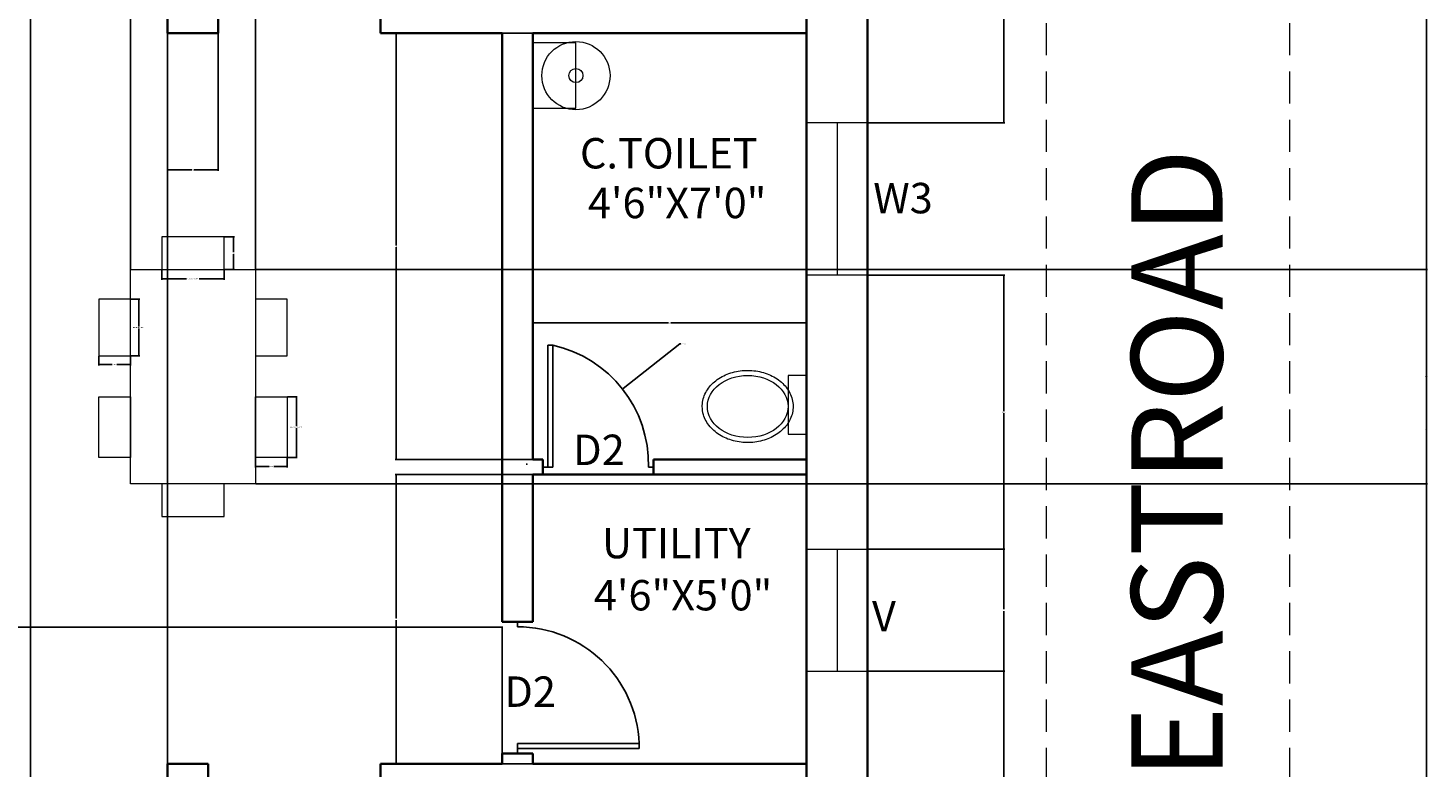
# Model space of a CAD drawing. Units: inches. Extents: x 2906 to 3403, y 1614 to 2150.
# Tile 3 of 4: x 3127 to 3403, y 1814 to 1960. Entities that reach past the tile are written whole.
import ezdxf

# ---------------------------------------------------------------- set-up
doc = ezdxf.new("R2010")
doc.units = ezdxf.units.IN
doc.linetypes.add('DASHED2', pattern=[9.525, 6.35, -3.175])
for name, color, linetype, lineweight in [('A-ANNO-DIMS', 2, 'Continuous', 18), ('A-ANNO-TEXT', 220, 'Continuous', 18), ('A-AREA-IDEN', 220, 'Continuous', 25), ('A-DOOR', 40, 'Continuous', 25), ('A-FLOR-FIXT', 121, 'Continuous', 18), ('A-FURN', 121, 'Continuous', 18), ('A-GLAZ', 2, 'Continuous', 18), ('A-WALL', 191, 'Continuous', 35), ('C-ROAD', 255, 'DASHED2', 18)]:
    doc.layers.add(name, color=color, linetype=linetype, lineweight=lineweight)
doc.styles.get("Standard").update_dxf_attribs({"font": 'arial.ttf'})
doc.dimstyles.get("Standard").update_dxf_attribs({"dimtxt": 0.18, "dimasz": 0.18, "dimexe": 0.18, "dimexo": 0.0625, "dimgap": 0.09, "dimtad": 0, "dimtih": 1, "dimtoh": 1, "dimdec": 4, "dimzin": 0, "dimdsep": 46, "dimtxsty": 'Standard', "dimcen": 0.09, "dimadec": 0, "dimazin": 0, "dimtfac": 1, "dimtdec": 4, "dimtofl": 0, "dimtmove": 0, "dimatfit": 3, "dimfxl": 1, "dimtolj": 1, "dimtzin": 0, "dimarcsym": 0})

# ---------------------------------------------------------------- blocks, each defined once
blk = doc.blocks.new('WINDOW-30')
for p, q in [((0, 12), (0, 0)), ((30, 12), (30, 0)), ((0, 6), (30, 6))]:
    blk.add_line(p, q)
blk = doc.blocks.new('WC-FLOOR')
blk.add_lwpolyline([(20.57, 13.25), (16.9, 13.25), (16.9, 1.66), (20.57, 1.66)], close=True)
blk.add_ellipse((8.95, 7.12), major_axis=(-7.95, 0), ratio=0.769471)
blk.add_open_spline([(0, 7.12), (0, 6.57), (0.08, 6.02), (0.48, 4.65), (0.93, 3.84), (2.12, 2.43), (2.86, 1.82), (4.56, 0.85), (5.51, 0.49), (7.5, 0.04), (8.54, -0.04), (10.6, 0.07), (11.62, 0.27), (13.52, 0.93), (14.4, 1.4), (15.92, 2.56), (16.56, 3.25), (17.49, 4.8), (17.78, 5.66), (17.96, 7.41), (17.85, 8.3), (17.23, 9.97), (16.74, 10.74), (15.46, 12.09), (14.67, 12.67), (12.92, 13.56), (11.94, 13.88), (9.93, 14.24), (8.88, 14.28), (6.83, 14.08), (5.83, 13.84), (3.97, 13.1), (3.12, 12.59), (1.68, 11.37), (1.09, 10.64), (0.26, 9.05), (0.03, 8.17), (0, 7.24), (0, 7.18), (0, 7.12)], degree=3, knots=[0, 0, 0, 0, 0.221105, 0.221105, 0.576279, 0.576279, 0.931454, 0.931454, 1.286628, 1.286628, 1.641803, 1.641803, 1.996977, 1.996977, 2.352152, 2.352152, 2.707326, 2.707326, 3.062501, 3.062501, 3.417675, 3.417675, 3.77285, 3.77285, 4.128024, 4.128024, 4.483198, 4.483198, 4.838373, 4.838373, 5.193547, 5.193547, 5.548722, 5.548722, 5.903896, 5.903896, 6.259071, 6.259071, 6.283185, 6.283185, 6.283185, 6.283185])
blk = doc.blocks.new('LAVATORY-WALL')
blk.add_lwpolyline([(15.24, 13.17), (6.72, 13.17), (6.72, 0.27), (15.24, 0.27)], close=True)
for radius in [6.72, 1.39]:
    blk.add_circle((6.72, 6.72), radius)
blk = doc.blocks.new('DINING-CHAIR-END')
blk.add_lwpolyline([(0, 0), (12.31, 0), (12.31, 6.47), (0, 6.47)], close=True)
blk = doc.blocks.new('DINING-CHAIR-SIDE-A')
blk.add_lwpolyline([(6.24, 11.19), (0, 11.19), (0, 0), (6.24, 0)], close=True)
blk = doc.blocks.new('DINING-CHAIR-SIDE-B')
blk.add_lwpolyline([(6.24, 0), (0, 0), (0, 11.97), (6.24, 11.97)], close=True)
blk = doc.blocks.new('*D34')
at = {"layer": 'A-ANNO-DIMS', "color": 0, "lineweight": -2, "transparency": 16777216}
for p, q in [((3153.49, 1912.61), (3153.49, 1910.65)), ((3153.67, 1910.83), (3158.4, 1910.83)), ((3165.63, 1910.83), (3160.9, 1910.83)), ((3165.81, 1912.61), (3165.81, 1910.65))]:
    blk.add_line(p, q, dxfattribs=at)
at = {"layer": 'A-ANNO-DIMS', "color": 0, "transparency": 16777216}
for points in [[(3153.67, 1910.86), (3153.67, 1910.8), (3153.49, 1910.83)], [(3165.63, 1910.86), (3165.63, 1910.8), (3165.81, 1910.83)]]:
    blk.add_solid(points, dxfattribs=at)
at = {"layer": 'Defpoints', "color": 0, "transparency": 16777216}
for p in [(3153.49, 1912.68), (3165.81, 1912.68), (3165.81, 1910.83)]:
    blk.add_point(p, dxfattribs=at)
at = {"layer": 'A-ANNO-DIMS', "color": 0, "transparency": 16777216, "insert": (3159.65, 1910.83), "char_height": 0.18, "attachment_point": 5}
blk.add_mtext('\\A1;END CHAIR 12 TYP.', dxfattribs=at)
blk = doc.blocks.new('*D35')
at = {"layer": 'A-ANNO-DIMS', "color": 0, "lineweight": -2, "transparency": 16777216}
for p, q in [((3165.87, 1919.15), (3167.83, 1919.15)), ((3167.65, 1918.97), (3167.65, 1916.1)), ((3167.65, 1912.86), (3167.65, 1915.73)), ((3165.87, 1912.68), (3167.83, 1912.68))]:
    blk.add_line(p, q, dxfattribs=at)
at = {"layer": 'A-ANNO-DIMS', "color": 0, "transparency": 16777216}
for points in [[(3167.62, 1918.97), (3167.68, 1918.97), (3167.65, 1919.15)], [(3167.62, 1912.86), (3167.68, 1912.86), (3167.65, 1912.68)]]:
    blk.add_solid(points, dxfattribs=at)
at = {"layer": 'Defpoints', "color": 0, "transparency": 16777216}
for p in [(3165.81, 1919.15), (3167.65, 1919.15), (3165.81, 1912.68)]:
    blk.add_point(p, dxfattribs=at)
at = {"layer": 'A-ANNO-DIMS', "color": 0, "transparency": 16777216, "insert": (3167.65, 1915.91), "char_height": 0.18, "attachment_point": 5}
blk.add_mtext('\\A1;6 TYP.', dxfattribs=at)
blk = doc.blocks.new('*D36')
at = {"layer": 'A-ANNO-DIMS', "color": 0, "lineweight": -2, "transparency": 16777216}
for p, q in [((3147.39, 1906.84), (3149.18, 1906.84)), ((3149, 1906.66), (3149, 1901.43)), ((3149, 1895.83), (3149, 1901.06)), ((3147.39, 1895.65), (3149.18, 1895.65))]:
    blk.add_line(p, q, dxfattribs=at)
at = {"layer": 'A-ANNO-DIMS', "color": 0, "transparency": 16777216}
for points in [[(3148.97, 1906.66), (3149.03, 1906.66), (3149, 1906.84)], [(3148.97, 1895.83), (3149.03, 1895.83), (3149, 1895.65)]]:
    blk.add_solid(points, dxfattribs=at)
at = {"layer": 'Defpoints', "color": 0, "transparency": 16777216}
for p in [(3147.32, 1906.84), (3149, 1906.84), (3147.32, 1895.65)]:
    blk.add_point(p, dxfattribs=at)
at = {"layer": 'A-ANNO-DIMS', "color": 0, "transparency": 16777216, "insert": (3149, 1901.25), "char_height": 0.18, "attachment_point": 5}
blk.add_mtext('\\A1;SIDE CHAIR A 11 TYP.', dxfattribs=at)
blk = doc.blocks.new('*D37')
at = {"layer": 'A-ANNO-DIMS', "color": 0, "lineweight": -2, "transparency": 16777216}
for p, q in [((3141.08, 1895.59), (3141.08, 1893.79)), ((3141.26, 1893.97), (3143.75, 1893.97)), ((3147.14, 1893.97), (3144.66, 1893.97)), ((3147.32, 1895.59), (3147.32, 1893.79))]:
    blk.add_line(p, q, dxfattribs=at)
at = {"layer": 'A-ANNO-DIMS', "color": 0, "transparency": 16777216}
for points in [[(3141.26, 1894), (3141.26, 1893.94), (3141.08, 1893.97)], [(3147.14, 1894), (3147.14, 1893.94), (3147.32, 1893.97)]]:
    blk.add_solid(points, dxfattribs=at)
at = {"layer": 'Defpoints', "color": 0, "transparency": 16777216}
for p in [(3141.08, 1895.65), (3147.32, 1895.65), (3147.32, 1893.97)]:
    blk.add_point(p, dxfattribs=at)
at = {"layer": 'A-ANNO-DIMS', "color": 0, "transparency": 16777216, "insert": (3144.2, 1893.97), "char_height": 0.18, "attachment_point": 5}
blk.add_mtext('\\A1;6 TYP.', dxfattribs=at)
blk = doc.blocks.new('*D38')
at = {"layer": 'A-ANNO-DIMS', "color": 0, "lineweight": -2, "transparency": 16777216}
for p, q in [((3178.3, 1887.61), (3180.22, 1887.61)), ((3180.04, 1887.43), (3180.04, 1881.8)), ((3180.04, 1875.81), (3180.04, 1881.44)), ((3178.3, 1875.63), (3180.22, 1875.63))]:
    blk.add_line(p, q, dxfattribs=at)
at = {"layer": 'A-ANNO-DIMS', "color": 0, "transparency": 16777216}
for points in [[(3180.01, 1887.43), (3180.07, 1887.43), (3180.04, 1887.61)], [(3180.01, 1875.81), (3180.07, 1875.81), (3180.04, 1875.63)]]:
    blk.add_solid(points, dxfattribs=at)
at = {"layer": 'Defpoints', "color": 0, "transparency": 16777216}
for p in [(3178.24, 1887.61), (3180.04, 1887.61), (3178.24, 1875.63)]:
    blk.add_point(p, dxfattribs=at)
at = {"layer": 'A-ANNO-DIMS', "color": 0, "transparency": 16777216, "insert": (3180.04, 1881.62), "char_height": 0.18, "attachment_point": 5}
blk.add_mtext('\\A1;SIDE CHAIR B 12 TYP.', dxfattribs=at)
blk = doc.blocks.new('*D39')
at = {"layer": 'A-ANNO-DIMS', "color": 0, "lineweight": -2, "transparency": 16777216}
for p, q in [((3172, 1875.57), (3172, 1873.66)), ((3178.24, 1875.57), (3178.24, 1873.66)), ((3172.18, 1873.84), (3174.66, 1873.84)), ((3178.06, 1873.84), (3175.58, 1873.84))]:
    blk.add_line(p, q, dxfattribs=at)
at = {"layer": 'A-ANNO-DIMS', "color": 0, "transparency": 16777216}
for points in [[(3172.18, 1873.87), (3172.18, 1873.81), (3172, 1873.84)], [(3178.06, 1873.87), (3178.06, 1873.81), (3178.24, 1873.84)]]:
    blk.add_solid(points, dxfattribs=at)
at = {"layer": 'Defpoints', "color": 0, "transparency": 16777216}
for p in [(3172, 1875.63), (3178.24, 1875.63), (3178.24, 1873.84)]:
    blk.add_point(p, dxfattribs=at)
at = {"layer": 'A-ANNO-DIMS', "color": 0, "transparency": 16777216, "insert": (3175.12, 1873.84), "char_height": 0.18, "attachment_point": 5}
blk.add_mtext('\\A1;6 TYP.', dxfattribs=at)
blk = doc.blocks.new('*D41')
at = {"layer": 'A-ANNO-DIMS', "color": 0, "lineweight": -2, "transparency": 16777216}
for p, q in [((3292.7, 2121.25), (3403.01, 2121.25)), ((3402.83, 2121.07), (3402.83, 1881.44)), ((3402.83, 1641.43), (3402.83, 1881.07)), ((3292.7, 1641.25), (3403.01, 1641.25))]:
    blk.add_line(p, q, dxfattribs=at)
at = {"layer": 'A-ANNO-DIMS', "color": 0, "transparency": 16777216}
for points in [[(3402.8, 2121.07), (3402.86, 2121.07), (3402.83, 2121.25)], [(3402.8, 1641.43), (3402.86, 1641.43), (3402.83, 1641.25)]]:
    blk.add_solid(points, dxfattribs=at)
at = {"layer": 'Defpoints', "color": 0, "transparency": 16777216}
for p in [(3292.63, 2121.25), (3402.83, 2121.25), (3292.63, 1641.25)]:
    blk.add_point(p, dxfattribs=at)
at = {"layer": 'A-ANNO-DIMS', "color": 0, "transparency": 16777216, "insert": (3402.83, 1881.25), "char_height": 0.18, "attachment_point": 5}
blk.add_mtext('\\A1;480', dxfattribs=at)
blk = doc.blocks.new('*D59')
at = {"layer": 'A-ANNO-DIMS', "color": 0, "lineweight": -2, "transparency": 16777216}
for p, q in [((3226.63, 1875.32), (3226.63, 1902.33)), ((3226.81, 1902.15), (3253.41, 1902.15)), ((3280.45, 1902.15), (3253.85, 1902.15)), ((3280.63, 1875.32), (3280.63, 1902.33))]:
    blk.add_line(p, q, dxfattribs=at)
at = {"layer": 'A-ANNO-DIMS', "color": 0, "transparency": 16777216}
for points in [[(3226.81, 1902.18), (3226.81, 1902.12), (3226.63, 1902.15)], [(3280.45, 1902.18), (3280.45, 1902.12), (3280.63, 1902.15)]]:
    blk.add_solid(points, dxfattribs=at)
at = {"layer": 'Defpoints', "color": 0, "transparency": 16777216}
for p in [(3280.63, 1902.15), (3226.63, 1875.25), (3280.63, 1875.25)]:
    blk.add_point(p, dxfattribs=at)
at = {"layer": 'A-ANNO-DIMS', "color": 0, "transparency": 16777216, "insert": (3253.63, 1902.15), "char_height": 0.18, "attachment_point": 5}
blk.add_mtext('\\A1;54', dxfattribs=at)
blk = doc.blocks.new('*D62')
at = {"layer": 'A-ANNO-DIMS', "color": 0, "lineweight": -2, "transparency": 16777216}
for p, q in [((3226.57, 1872.25), (3199.55, 1872.25)), ((3199.73, 1872.07), (3199.73, 1843.94)), ((3199.73, 1815.43), (3199.73, 1843.57)), ((3226.57, 1815.25), (3199.55, 1815.25))]:
    blk.add_line(p, q, dxfattribs=at)
at = {"layer": 'A-ANNO-DIMS', "color": 0, "transparency": 16777216}
for points in [[(3199.7, 1872.07), (3199.76, 1872.07), (3199.73, 1872.25)], [(3199.7, 1815.43), (3199.76, 1815.43), (3199.73, 1815.25)]]:
    blk.add_solid(points, dxfattribs=at)
at = {"layer": 'Defpoints', "color": 0, "transparency": 16777216}
for p in [(3199.73, 1872.25), (3226.63, 1872.25), (3226.63, 1815.25)]:
    blk.add_point(p, dxfattribs=at)
at = {"layer": 'A-ANNO-DIMS', "color": 0, "transparency": 16777216, "insert": (3199.73, 1843.75), "char_height": 0.18, "attachment_point": 5}
blk.add_mtext('\\A1;57', dxfattribs=at)
blk = doc.blocks.new('*D63')
at = {"layer": 'A-ANNO-DIMS', "color": 0, "lineweight": -2, "transparency": 16777216}
for p, q in [((3226.57, 1959.25), (3199.55, 1959.25)), ((3199.73, 1959.07), (3199.73, 1917.44)), ((3199.73, 1875.43), (3199.73, 1917.07)), ((3226.57, 1875.25), (3199.55, 1875.25))]:
    blk.add_line(p, q, dxfattribs=at)
at = {"layer": 'A-ANNO-DIMS', "color": 0, "transparency": 16777216}
for points in [[(3199.7, 1959.07), (3199.76, 1959.07), (3199.73, 1959.25)], [(3199.7, 1875.43), (3199.76, 1875.43), (3199.73, 1875.25)]]:
    blk.add_solid(points, dxfattribs=at)
at = {"layer": 'Defpoints', "color": 0, "transparency": 16777216}
for p in [(3199.73, 1959.25), (3226.63, 1959.25), (3226.63, 1875.25)]:
    blk.add_point(p, dxfattribs=at)
at = {"layer": 'A-ANNO-DIMS', "color": 0, "transparency": 16777216, "insert": (3199.73, 1917.25), "char_height": 0.18, "attachment_point": 5}
blk.add_mtext('\\A1;84', dxfattribs=at)
blk = doc.blocks.new('*D65')
at = {"layer": 'A-ANNO-DIMS', "color": 0, "lineweight": -2, "transparency": 16777216}
for p, q in [((2944.63, 1815.32), (2944.63, 1842.33)), ((2944.81, 1842.15), (3082.34, 1842.15)), ((3220.45, 1842.15), (3082.92, 1842.15)), ((3220.63, 1815.32), (3220.63, 1842.33))]:
    blk.add_line(p, q, dxfattribs=at)
at = {"layer": 'A-ANNO-DIMS', "color": 0, "transparency": 16777216}
for points in [[(2944.81, 1842.18), (2944.81, 1842.12), (2944.63, 1842.15)], [(3220.45, 1842.18), (3220.45, 1842.12), (3220.63, 1842.15)]]:
    blk.add_solid(points, dxfattribs=at)
at = {"layer": 'Defpoints', "color": 0, "transparency": 16777216}
for p in [(3220.63, 1842.15), (2944.63, 1815.25), (3220.63, 1815.25)]:
    blk.add_point(p, dxfattribs=at)
at = {"layer": 'A-ANNO-DIMS', "color": 0, "transparency": 16777216, "insert": (3082.63, 1842.15), "char_height": 0.18, "attachment_point": 5}
blk.add_mtext('\\A1;276', dxfattribs=at)
blk = doc.blocks.new('*D66')
at = {"layer": 'A-ANNO-DIMS', "color": 0, "lineweight": -2, "transparency": 16777216}
for p, q in [((3292.7, 2121.25), (3319.71, 2121.25)), ((3319.53, 2121.07), (3319.53, 2031.6)), ((3319.53, 1941.76), (3319.53, 2031.24)), ((3292.7, 1941.58), (3319.71, 1941.58))]:
    blk.add_line(p, q, dxfattribs=at)
at = {"layer": 'A-ANNO-DIMS', "color": 0, "transparency": 16777216}
for points in [[(3319.5, 2121.07), (3319.56, 2121.07), (3319.53, 2121.25)], [(3319.5, 1941.76), (3319.56, 1941.76), (3319.53, 1941.58)]]:
    blk.add_solid(points, dxfattribs=at)
at = {"layer": 'Defpoints', "color": 0, "transparency": 16777216}
for p in [(3292.63, 2121.25), (3292.63, 1941.58), (3319.53, 1941.58)]:
    blk.add_point(p, dxfattribs=at)
at = {"layer": 'A-ANNO-DIMS', "color": 0, "transparency": 16777216, "insert": (3319.53, 2031.42), "char_height": 0.18, "attachment_point": 5}
blk.add_mtext('\\A1;179.67', dxfattribs=at)
blk = doc.blocks.new('*D67')
at = {"layer": 'A-ANNO-DIMS', "color": 0, "lineweight": -2, "transparency": 16777216}
for p, q in [((3292.7, 1911.58), (3319.71, 1911.58)), ((3319.53, 1911.4), (3319.53, 1884.74)), ((3319.53, 1857.71), (3319.53, 1884.37)), ((3292.7, 1857.53), (3319.71, 1857.53))]:
    blk.add_line(p, q, dxfattribs=at)
at = {"layer": 'A-ANNO-DIMS', "color": 0, "transparency": 16777216}
for points in [[(3319.5, 1911.4), (3319.56, 1911.4), (3319.53, 1911.58)], [(3319.5, 1857.71), (3319.56, 1857.71), (3319.53, 1857.53)]]:
    blk.add_solid(points, dxfattribs=at)
at = {"layer": 'Defpoints', "color": 0, "transparency": 16777216}
for p in [(3292.63, 1911.58), (3292.63, 1857.53), (3319.53, 1857.53)]:
    blk.add_point(p, dxfattribs=at)
at = {"layer": 'A-ANNO-DIMS', "color": 0, "transparency": 16777216, "insert": (3319.53, 1884.56), "char_height": 0.18, "attachment_point": 5}
blk.add_mtext('\\A1;54.05', dxfattribs=at)
blk = doc.blocks.new('*D68')
at = {"layer": 'A-ANNO-DIMS', "color": 0, "lineweight": -2, "transparency": 16777216}
for p, q in [((3292.7, 1857.53), (3319.71, 1857.53)), ((3319.53, 1857.35), (3319.53, 1845.71)), ((3319.53, 1833.71), (3319.53, 1845.35)), ((3292.7, 1833.53), (3319.71, 1833.53))]:
    blk.add_line(p, q, dxfattribs=at)
at = {"layer": 'A-ANNO-DIMS', "color": 0, "transparency": 16777216}
for points in [[(3319.5, 1857.35), (3319.56, 1857.35), (3319.53, 1857.53)], [(3319.5, 1833.71), (3319.56, 1833.71), (3319.53, 1833.53)]]:
    blk.add_solid(points, dxfattribs=at)
at = {"layer": 'Defpoints', "color": 0, "transparency": 16777216}
for p in [(3292.63, 1857.53), (3292.63, 1833.53), (3319.53, 1833.53)]:
    blk.add_point(p, dxfattribs=at)
at = {"layer": 'A-ANNO-DIMS', "color": 0, "transparency": 16777216, "insert": (3319.53, 1845.53), "char_height": 0.18, "attachment_point": 5}
blk.add_mtext('\\A1;24', dxfattribs=at)
blk = doc.blocks.new('*D69')
at = {"layer": 'A-ANNO-DIMS', "color": 0, "lineweight": -2, "transparency": 16777216}
for p, q in [((3292.7, 1833.53), (3319.71, 1833.53)), ((3319.53, 1833.35), (3319.53, 1804.89)), ((3319.53, 1776.07), (3319.53, 1804.53)), ((3292.7, 1775.89), (3319.71, 1775.89))]:
    blk.add_line(p, q, dxfattribs=at)
at = {"layer": 'A-ANNO-DIMS', "color": 0, "transparency": 16777216}
for points in [[(3319.5, 1833.35), (3319.56, 1833.35), (3319.53, 1833.53)], [(3319.5, 1776.07), (3319.56, 1776.07), (3319.53, 1775.89)]]:
    blk.add_solid(points, dxfattribs=at)
at = {"layer": 'Defpoints', "color": 0, "transparency": 16777216}
for p in [(3292.63, 1833.53), (3292.63, 1775.89), (3319.53, 1775.89)]:
    blk.add_point(p, dxfattribs=at)
at = {"layer": 'A-ANNO-DIMS', "color": 0, "transparency": 16777216, "insert": (3319.53, 1804.71), "char_height": 0.18, "attachment_point": 5}
blk.add_mtext('\\A1;57.63', dxfattribs=at)
blk = doc.blocks.new('*D72')
at = {"layer": 'A-ANNO-DIMS', "color": 0, "lineweight": -2, "transparency": 16777216}
for p, q in [((3154.63, 1959.19), (3154.63, 1932.17)), ((3164.63, 1959.19), (3164.63, 1932.17)), ((3154.81, 1932.35), (3159.42, 1932.35)), ((3164.45, 1932.35), (3159.84, 1932.35))]:
    blk.add_line(p, q, dxfattribs=at)
at = {"layer": 'A-ANNO-DIMS', "color": 0, "transparency": 16777216}
for points in [[(3154.81, 1932.38), (3154.81, 1932.32), (3154.63, 1932.35)], [(3164.45, 1932.38), (3164.45, 1932.32), (3164.63, 1932.35)]]:
    blk.add_solid(points, dxfattribs=at)
at = {"layer": 'Defpoints', "color": 0, "transparency": 16777216}
for p in [(3154.63, 1959.25), (3164.63, 1959.25), (3154.63, 1932.35)]:
    blk.add_point(p, dxfattribs=at)
at = {"layer": 'A-ANNO-DIMS', "color": 0, "transparency": 16777216, "insert": (3159.63, 1932.35), "char_height": 0.18, "attachment_point": 5}
blk.add_mtext('\\A1;10', dxfattribs=at)
blk = doc.blocks.new('*D75')
at = {"layer": 'A-ANNO-DIMS', "color": 0, "lineweight": -2, "transparency": 16777216}
for p, q in [((3127.63, 2013.19), (3127.63, 1613.51)), ((3154.63, 2013.19), (3154.63, 1613.51)), ((3127.81, 1613.69), (3140.91, 1613.69)), ((3154.45, 1613.69), (3141.35, 1613.69))]:
    blk.add_line(p, q, dxfattribs=at)
at = {"layer": 'A-ANNO-DIMS', "color": 0, "transparency": 16777216}
for points in [[(3127.81, 1613.72), (3127.81, 1613.66), (3127.63, 1613.69)], [(3154.45, 1613.72), (3154.45, 1613.66), (3154.63, 1613.69)]]:
    blk.add_solid(points, dxfattribs=at)
at = {"layer": 'Defpoints', "color": 0, "transparency": 16777216}
for p in [(3127.63, 2013.25), (3154.63, 2013.25), (3154.63, 1613.69)]:
    blk.add_point(p, dxfattribs=at)
at = {"layer": 'A-ANNO-DIMS', "color": 0, "transparency": 16777216, "insert": (3141.13, 1613.69), "char_height": 0.18, "attachment_point": 5}
blk.add_mtext('\\A1;27', dxfattribs=at)
blk = doc.blocks.new('*D78')
at = {"layer": 'A-ANNO-DIMS', "color": 0, "lineweight": -2, "transparency": 16777216}
for p, q in [((3147.32, 1912.74), (3147.32, 2149.96)), ((3147.5, 2149.78), (3159.2, 2149.78)), ((3171.82, 2149.78), (3160.13, 2149.78)), ((3172, 1912.74), (3172, 2149.96))]:
    blk.add_line(p, q, dxfattribs=at)
at = {"layer": 'A-ANNO-DIMS', "color": 0, "transparency": 16777216}
for points in [[(3147.5, 2149.81), (3147.5, 2149.75), (3147.32, 2149.78)], [(3171.82, 2149.81), (3171.82, 2149.75), (3172, 2149.78)]]:
    blk.add_solid(points, dxfattribs=at)
at = {"layer": 'Defpoints', "color": 0, "transparency": 16777216}
for p in [(3172, 2149.78), (3147.32, 1912.68), (3172, 1912.68)]:
    blk.add_point(p, dxfattribs=at)
at = {"layer": 'A-ANNO-DIMS', "color": 0, "transparency": 16777216, "insert": (3159.66, 2149.78), "char_height": 0.18, "attachment_point": 5}
blk.add_mtext('\\A1;24.675', dxfattribs=at)
blk = doc.blocks.new('*D79')
at = {"layer": 'A-ANNO-DIMS', "color": 0, "lineweight": -2, "transparency": 16777216}
for p, q in [((3172.06, 1912.68), (3403.01, 1912.68)), ((3402.83, 1912.5), (3402.83, 1891.75)), ((3402.83, 1870.64), (3402.83, 1891.39)), ((3172.06, 1870.46), (3403.01, 1870.46))]:
    blk.add_line(p, q, dxfattribs=at)
at = {"layer": 'A-ANNO-DIMS', "color": 0, "transparency": 16777216}
for points in [[(3402.8, 1912.5), (3402.86, 1912.5), (3402.83, 1912.68)], [(3402.8, 1870.64), (3402.86, 1870.64), (3402.83, 1870.46)]]:
    blk.add_solid(points, dxfattribs=at)
at = {"layer": 'Defpoints', "color": 0, "transparency": 16777216}
for p in [(3172, 1912.68), (3402.83, 1912.68), (3172, 1870.46)]:
    blk.add_point(p, dxfattribs=at)
at = {"layer": 'A-ANNO-DIMS', "color": 0, "transparency": 16777216, "insert": (3402.83, 1891.57), "char_height": 0.18, "attachment_point": 5}
blk.add_mtext('\\A1;42.22', dxfattribs=at)
blk = doc.blocks.new('*D83')
at = {"layer": 'A-ANNO-DIMS', "color": 0, "lineweight": -2, "transparency": 16777216}
for p, q in [((3255.67, 1898.01), (3244.48, 1889.24)), ((3255.85, 1898.01), (3255.67, 1898.01)), ((3225.36, 1874.32), (3225.54, 1874.32)), ((3225.45, 1874.23), (3225.45, 1874.41))]:
    blk.add_line(p, q, dxfattribs=at)
at = {"layer": 'A-ANNO-DIMS', "color": 0, "transparency": 16777216}
blk.add_solid([(3244.46, 1889.26), (3244.5, 1889.21), (3244.34, 1889.13)], dxfattribs=at)
at = {"layer": 'Defpoints', "color": 0, "transparency": 16777216}
for p in [(3244.34, 1889.13), (3225.45, 1874.32)]:
    blk.add_point(p, dxfattribs=at)
at = {"layer": 'A-ANNO-DIMS', "color": 0, "transparency": 16777216, "insert": (3256.35, 1898.01), "char_height": 0.18, "attachment_point": 5}
blk.add_mtext('\\A1;2X R24', dxfattribs=at)

msp = doc.modelspace()

# ---------------------------------------------------------------- linework, layer by layer
at = {"layer": 'A-DOOR'}
for p, q in [((3229.6325, 1873.754), (3229.6325, 1897.754)), ((3229.6325, 1897.754), (3230.6325, 1897.754)), ((3230.6325, 1897.754), (3230.6325, 1873.754)), ((3228.6325, 1873.754), (3229.6325, 1873.754)), ((3230.6325, 1873.754), (3229.6325, 1873.754)), ((3250.4461, 1873.754), (3249.4461, 1873.754)), ((3223.6325, 1843.254), (3223.6325, 1842.254)), ((3247.6325, 1819.254), (3223.6325, 1819.254)), ((3223.6325, 1819.254), (3223.6325, 1818.254)), ((3247.6325, 1818.254), (3247.6325, 1819.254)), ((3223.6325, 1817.254), (3223.6325, 1818.254)), ((3223.6325, 1818.254), (3247.6325, 1818.254))]:
    msp.add_line(p, q, dxfattribs=at)
for centre, start, end in [((3225.4528, 1874.3196), 358.649577, 77.536279), ((3223.6534, 1818.254), 2.387994, 90.049757)]:
    msp.add_arc(centre, 24, start, end, dxfattribs=at)
at = {"layer": 'A-FURN'}
msp.add_lwpolyline([(3147.3239, 1912.6757), (3171.9988, 1912.6757), (3171.9988, 1870.4563), (3147.3239, 1870.4563)], close=True, dxfattribs=at)
at = {"layer": 'A-GLAZ'}
for p, q in [((3280.6325, 1857.5286), (3292.6325, 1857.5286)), ((3286.6325, 1857.5286), (3286.6325, 1833.5286)), ((3280.6325, 1833.5286), (3292.6325, 1833.5286))]:
    msp.add_line(p, q, dxfattribs=at)
at = {"layer": 'A-WALL'}
for p, q in [((3280.6325, 2109.254), (3280.6325, 1701.254)), ((3154.6325, 1959.254), (3154.6325, 2013.254)), ((3164.6325, 1965.254), (3164.6325, 1959.254)), ((3196.6325, 1965.254), (3196.6325, 1959.254)), ((3154.6325, 1959.254), (3164.6325, 1959.254)), ((3196.6325, 1959.254), (3220.6325, 1959.254)), ((3220.6325, 1959.254), (3220.6325, 1843.254)), ((3226.6325, 1959.254), (3226.6325, 1875.254)), ((3226.6325, 1959.254), (3280.6325, 1959.254)), ((3226.6325, 1875.254), (3228.6325, 1875.254)), ((3226.6325, 1875.254), (3228.6325, 1875.254)), ((3228.6325, 1875.254), (3228.6325, 1872.254)), ((3250.4461, 1875.254), (3280.6325, 1875.254)), ((3250.4461, 1875.254), (3250.4461, 1872.254)), ((3226.6325, 1872.254), (3228.6325, 1872.254)), ((3226.6325, 1872.254), (3226.6325, 1843.254)), ((3228.6325, 1872.254), (3280.6325, 1872.254)), ((3220.6325, 1843.254), (3226.6325, 1843.254)), ((3220.6325, 1815.254), (3220.6325, 1817.254)), ((3220.6325, 1817.254), (3226.6325, 1817.254)), ((3220.6325, 1817.254), (3220.6325, 1815.254)), ((3226.6325, 1817.254), (3226.6325, 1815.254)), ((3154.6325, 1653.254), (3154.6325, 1815.254)), ((3154.6325, 1815.254), (3162.6325, 1815.254)), ((3162.6325, 1809.254), (3162.6325, 1815.254)), ((3196.6325, 1809.254), (3196.6325, 1815.254)), ((3196.6325, 1815.254), (3220.6325, 1815.254)), ((3226.6325, 1815.254), (3280.6325, 1815.254))]:
    msp.add_line(p, q, dxfattribs=at)
msp.add_lwpolyline([(3022.1668, 1641.254), (2932.6325, 1641.254), (2932.6325, 2121.254), (3292.6325, 2121.254), (3292.6325, 1689.254)], dxfattribs=at)
at = {"layer": 'C-ROAD'}
for p, q in [((3327.9288, 1640.586), (3327.9288, 2122.8771)), ((3375.9288, 1640.586), (3375.9288, 2122.8771))]:
    msp.add_line(p, q, dxfattribs=at)

# ---------------------------------------------------------------- block references
at = {"layer": 'A-FLOR-FIXT', "rotation": 180}
msp.add_blockref('LAVATORY-WALL', (3241.874, 1957.6339), dxfattribs=at)
at = {"layer": 'A-FLOR-FIXT'}
msp.add_blockref('WC-FLOOR', (3260.066, 1878.57), dxfattribs=at)
at = {"layer": 'A-FURN'}
for name, p in [('DINING-CHAIR-END', (3153.493, 1912.676)), ('DINING-CHAIR-SIDE-A', (3141.084, 1895.653)), ('DINING-CHAIR-SIDE-A', (3171.9992, 1895.653)), ('DINING-CHAIR-SIDE-B', (3141.084, 1875.633)), ('DINING-CHAIR-SIDE-B', (3171.9992, 1875.633)), ('DINING-CHAIR-END', (3153.493, 1863.9815))]:
    msp.add_blockref(name, p, dxfattribs=at)
at = {"layer": 'A-GLAZ', "rotation": 269.999999999997}
msp.add_blockref('WINDOW-30', (3280.6326, 1941.5832), dxfattribs=at)

# ---------------------------------------------------------------- texts
at = {"layer": 'A-ANNO-TEXT'}
msp.add_attdef('EASTROAD', (3362.6272, 1812.1692), '', height=18, rotation=90, dxfattribs=at)
for tag, p in [('W3', (3293.7711, 1923.764)), ('D2', (3234.6019, 1874.1377)), ('V', (3293.5225, 1841.3544)), ('D2', (3221.0346, 1826.4659))]:
    msp.add_attdef(tag, p, '', height=6, dxfattribs=at)
at = {"layer": 'A-AREA-IDEN'}
for tag, p in [('C.TOILET', (3235.9462, 1932.6075)), ('4\'6"X7\'0"', (3237.5225, 1922.8079)), ('UTILITY', (3240.2999, 1855.7556)), ('4\'6"X5\'0"', (3238.6916, 1845.4797))]:
    msp.add_attdef(tag, p, '', height=6, dxfattribs=at)

# ---------------------------------------------------------------- dimensions: what is measured, and where the dimension line sits
at = {"layer": 'A-ANNO-DIMS'}
for base, p1, p2, override, picture, middle in [((3171.9988, 2149.7771), (3147.3239, 1912.6757), (3171.9988, 1912.6757), {"dimdec": 3, "dimlfac": 1, "dimrnd": 0, "dimzin": 0, "dimdsep": 46, "dimlunit": 2}, '*D78', (3159.6614, 2149.7771)), ((3154.6325, 1613.686), (3127.6325, 2013.254), (3154.6325, 2013.254), {"dimdec": 0, "dimlfac": 1, "dimrnd": 0, "dimzin": 0, "dimdsep": 46, "dimlunit": 2}, '*D75', (3141.1325, 1613.686)), ((3280.6325, 1902.154), (3226.6325, 1875.254), (3280.6325, 1875.254), {"dimdec": 0, "dimlfac": 1, "dimrnd": 0, "dimzin": 0, "dimdsep": 46, "dimlunit": 2}, '*D59', (3253.6325, 1902.154)), ((3220.6325, 1842.154), (2944.6325, 1815.254), (3220.6325, 1815.254), {"dimdec": 0, "dimlfac": 1, "dimrnd": 0, "dimzin": 0, "dimdsep": 46, "dimlunit": 2}, '*D65', (3082.6325, 1842.154))]:
    dim = msp.add_linear_dim(base=base, p1=p1, p2=p2, dimstyle='Standard', override=override, dxfattribs=at)
    dim.commit()
    dim.dimension.update_dxf_attribs({"geometry": picture, "text_midpoint": middle})
for base, p1, p2, angle, override, picture, middle in [((3402.8288, 2121.254), (3292.6325, 1641.254), (3292.6325, 2121.254), 90, {"dimdec": 0, "dimlfac": 1, "dimrnd": 0, "dimzin": 0, "dimdsep": 46, "dimlunit": 2}, '*D41', (3402.8288, 1881.254)), ((3319.5325, 1941.5831), (3292.6325, 2121.254), (3292.6325, 1941.5831), 270, {"dimdec": 2, "dimlfac": 1, "dimrnd": 0, "dimzin": 0, "dimdsep": 46, "dimlunit": 2}, '*D66', (3319.5325, 2031.4186)), ((3154.6325, 1932.354), (3164.6325, 1959.254), (3154.6325, 1959.254), 180, {"dimdec": 0, "dimlfac": 1, "dimrnd": 0, "dimzin": 0, "dimdsep": 46, "dimlunit": 2}, '*D72', (3159.6325, 1932.354)), ((3199.7325, 1959.254), (3226.6325, 1875.254), (3226.6325, 1959.254), 90, {"dimdec": 0, "dimlfac": 1, "dimrnd": 0, "dimzin": 0, "dimdsep": 46, "dimlunit": 2}, '*D63', (3199.7325, 1917.254)), ((3402.8288, 1912.6757), (3171.9988, 1870.4563), (3171.9988, 1912.6757), 90, {"dimdec": 2, "dimlfac": 1, "dimrnd": 0, "dimzin": 0, "dimdsep": 46, "dimlunit": 2}, '*D79', (3402.8288, 1891.566)), ((3319.5325, 1857.5286), (3292.6325, 1911.5831), (3292.6325, 1857.5286), 270, {"dimdec": 2, "dimlfac": 1, "dimrnd": 0, "dimzin": 0, "dimdsep": 46, "dimlunit": 2}, '*D67', (3319.5325, 1884.5559)), ((3199.7325, 1872.254), (3226.6325, 1815.254), (3226.6325, 1872.254), 90, {"dimdec": 0, "dimlfac": 1, "dimrnd": 0, "dimzin": 0, "dimdsep": 46, "dimlunit": 2}, '*D62', (3199.7325, 1843.754)), ((3319.5325, 1833.5286), (3292.6325, 1857.5286), (3292.6325, 1833.5286), 270, {"dimdec": 0, "dimlfac": 1, "dimrnd": 0, "dimzin": 0, "dimdsep": 46, "dimlunit": 2}, '*D68', (3319.5325, 1845.5286)), ((3319.5325, 1775.8947), (3292.6325, 1833.5286), (3292.6325, 1775.8947), 270, {"dimdec": 2, "dimlfac": 1, "dimrnd": 0, "dimzin": 0, "dimdsep": 46, "dimlunit": 2}, '*D69', (3319.5325, 1804.7116))]:
    dim = msp.add_linear_dim(base=base, p1=p1, p2=p2, angle=angle, dimstyle='Standard', override=override, dxfattribs=at)
    dim.commit()
    dim.dimension.update_dxf_attribs({"geometry": picture, "text_midpoint": middle})
for base, p1, p2, text, picture, middle in [((3167.654, 1919.1507), (3165.8069, 1912.6757), (3165.8069, 1919.1507), '<> TYP.', '*D35', (3167.654, 1915.9132)), ((3149.0021, 1906.8407), (3147.3239, 1895.6529), (3147.3239, 1906.8407), 'SIDE CHAIR A <> TYP.', '*D36', (3149.0021, 1901.2468)), ((3180.0351, 1887.6055), (3178.2391, 1875.6325), (3178.2391, 1887.6055), 'SIDE CHAIR B <> TYP.', '*D38', (3180.0351, 1881.619))]:
    dim = msp.add_linear_dim(base=base, p1=p1, p2=p2, angle=90, text=text, dimstyle='Standard', override={"dimdec": 0, "dimlfac": 1, "dimrnd": 0, "dimzin": 0, "dimdsep": 46, "dimlunit": 2}, dxfattribs=at)
    dim.commit()
    dim.dimension.update_dxf_attribs({"geometry": picture, "text_midpoint": middle})
for base, p1, p2, text, picture, middle in [((3165.8069, 1910.8286), (3153.4926, 1912.6757), (3165.8069, 1912.6757), 'END CHAIR <> TYP.', '*D34', (3159.6497, 1910.8286)), ((3147.3239, 1893.9747), (3141.0836, 1895.6529), (3147.3239, 1895.6529), '<> TYP.', '*D37', (3144.2037, 1893.9747)), ((3178.2391, 1873.8366), (3171.9988, 1875.6325), (3178.2391, 1875.6325), '<> TYP.', '*D39', (3175.119, 1873.8366))]:
    dim = msp.add_linear_dim(base=base, p1=p1, p2=p2, text=text, dimstyle='Standard', override={"dimdec": 0, "dimlfac": 1, "dimrnd": 0, "dimzin": 0, "dimdsep": 46, "dimlunit": 2}, dxfattribs=at)
    dim.commit()
    dim.dimension.update_dxf_attribs({"geometry": picture, "text_midpoint": middle})
dim = msp.add_radius_dim(center=(3225.4528, 1874.3196), mpoint=(3244.3411, 1889.1261), text='2X <>', dimstyle='Standard', override={"dimdec": 0, "dimlfac": 1, "dimrnd": 0, "dimzin": 0, "dimdsep": 46, "dimlunit": 2}, dxfattribs=at)
dim.commit()
dim.dimension.update_dxf_attribs({"geometry": '*D83', "text_midpoint": (3256.3537, 1898.01), "dimtype": 164})

doc.saveas('drawing.dxf')
